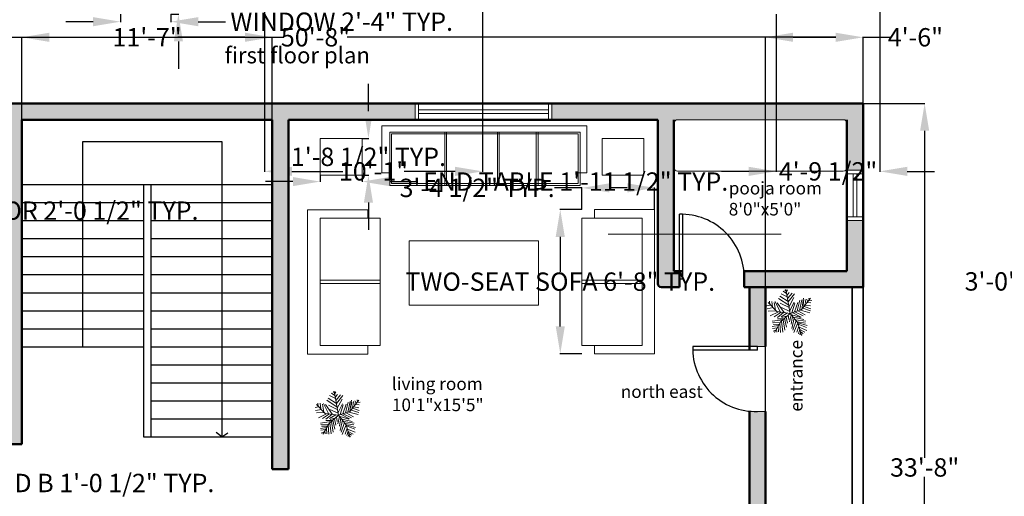
# Model space of a CAD drawing. Units: inches. Extents: x -2 to 7298, y -2 to 4583.
# Tile 3 of 6: x 6252 to 6799, y 3880 to 4144. Entities that reach past the tile are written whole.
import ezdxf

# ---------------------------------------------------------------- set-up
doc = ezdxf.new("R2010")
doc.units = ezdxf.units.IN
doc.header["$MEASUREMENT"] = 0
doc.linetypes.add('ACAD_ISO02W100', pattern=[15, 12, -3])
for name, color, linetype, lineweight in [('A-ANNO-DIMS', 2, 'Continuous', 18), ('A-ANNO-TEXT', 7, 'Continuous', 25), ('A-AREA-IDEN', 7, 'Continuous', 18), ('A-DOOR', 4, 'Continuous', 25), ('A-FLOR-CASE', 30, 'Continuous', 18), ('A-FLOR-STRS', 7, 'Continuous', 25), ('A-FURN', 8, 'Continuous', 18), ('A-GLAZ', 4, 'Continuous', 18), ('A-PLAN-REFR', 8, 'Continuous', 13), ('A-WALL', 7, 'Continuous', 50), ('A-WALL-HIDN', 7, 'ACAD_ISO02W100', 18), ('A-WALL-PATT', 18, 'Continuous', 13), ('C-PROP', 7, 'Continuous', 35), ('L-PLNT', 3, 'Continuous', 13)]:
    doc.layers.add(name, color=color, linetype=linetype, lineweight=lineweight)
doc.styles.get("Standard").update_dxf_attribs({"font": 'arial.ttf'})
doc.dimstyles.get("Standard").update_dxf_attribs({"dimtxt": 10.18, "dimasz": 15.18, "dimexe": 0.18, "dimexo": 0.0625, "dimgap": 0.09, "dimtad": 0, "dimtih": 1, "dimtoh": 1, "dimdec": 0, "dimzin": 0, "dimdsep": 46, "dimlunit": 3, "dimtxsty": 'Standard', "dimcen": 0.09, "dimadec": 0, "dimazin": 0, "dimtfac": 1, "dimtdec": 0, "dimtofl": 0, "dimtmove": 0, "dimatfit": 3, "dimfxl": 1, "dimtolj": 1, "dimtzin": 0, "dimarcsym": 0})

# ---------------------------------------------------------------- blocks, each defined once
blk = doc.blocks.new('*U11')
for p, q in [((-8.737, 47.138), (-17.069, 52.711)), ((-10.186, 53.64), (-13.084, 55.962)), ((0, 0), (-10.5, 57)), ((-9.099, 51.782), (-6.563, 55.962)), ((-7.65, 43.423), (-2.578, 49.46)), ((-5.839, 35.992), (4.667, 48.067)), ((-31.5, 4.5), (-52.5, 25.5)), ((-48.585, 21.131), (-49.309, 29.026)), ((-43.513, 28.561), (-42.427, 15.558)), ((-38.442, 26.239), (-34.819, 7.663)), ((-35.544, 28.097), (-24.314, 3.947)), ((-14.533, 2.09), (-30.834, 25.31)), ((-3.665, 19.273), (-27.574, 35.527)), ((-5.114, 28.097), (-24.676, 40.636)), ((-24.314, 23.917), (-2.941, 13.7)), ((-7.288, 39.707), (-21.778, 46.673)), ((-5.114, 27.632), (10.463, 46.673)), ((-2.941, 16.486), (8.652, 37.85)), ((-1.129, 6.734), (9.014, 26.704)), ((3.942, 1.625), (11.187, 24.381)), ((10.101, 3.483), (17.708, 26.239)), ((16.259, 5.805), (23.142, 31.348)), ((22.055, 7.198), (27.489, 32.277)), ((27, 9), (48, 36)), ((27.127, 9.056), (31.112, 35.992)), ((31.836, 30.883), (32.561, 16.486)), ((35.096, 32.741), (37.27, 22.524)), ((38.719, 34.134), (41.979, 28.561)), ((40.53, 25.775), (48.862, 24.846)), ((43.791, 29.954), (51.036, 30.883)), ((44.153, 36.456), (45.239, 32.741)), ((-47.498, 19.737), (-55.83, 18.344)), ((-40.615, 13.7), (-55.105, 10.913)), ((-33.37, 6.269), (-52.207, 5.34)), ((-28.299, 3.483), (-47.86, -5.805)), ((-21.416, 3.018), (-38.079, -8.128)), ((0, 0), (-31.5, 4.5)), ((-15.982, 2.09), (-30.11, -9.521)), ((0, 0), (-22.5, -19.5)), ((-6.563, 1.161), (-21.416, -8.128)), ((-20.691, 13.7), (-1.129, 4.876)), ((0, 0), (27, 9)), ((0, 0), (18, -22.5)), ((6.478, 1.625), (26.04, -8.592)), ((11.187, 3.483), (30.749, -5.805)), ((18.07, 5.805), (35.096, -3.483)), ((24.229, 7.663), (46.688, 1.625)), ((29.662, 12.307), (48.137, 6.269)), ((33.285, 16.486), (48.862, 10.913)), ((36.183, 19.737), (48.137, 17.88)), ((-17.431, -15.094), (-42.789, -18.809)), ((-24.314, -21.596), (-42.427, -22.06)), ((-22.5, -19.5), (-37.5, -45)), ((-15.257, -12.772), (-30.11, -12.772)), ((-20.691, -18.345), (-17.793, -44.352)), ((-6.563, -5.805), (-19.967, -9.985)), ((-17.069, -15.094), (-12.721, -40.172)), ((-13.446, -11.378), (-8.737, -32.741)), ((-9.461, -8.592), (-6.201, -23.453)), ((-4.752, -3.483), (-3.665, -14.629)), ((2.493, -3.019), (-1.491, -20.202)), ((1.769, -2.555), (24.229, -9.521)), ((5.029, -6.27), (2.131, -25.775)), ((9.014, -11.378), (3.58, -35.992)), ((14.085, -16.951), (6.478, -40.172)), ((7.565, -9.056), (32.198, -14.629)), ((18.07, -22.524), (8.289, -45.745)), ((12.274, -15.094), (36.907, -18.809)), ((16.259, -19.738), (36.183, -22.989)), ((18, -22.5), (27, -52.5)), ((18.433, -22.524), (40.53, -29.026)), ((-28.299, -29.026), (-42.789, -31.348)), ((-30.834, -34.135), (-42.427, -35.528)), ((-34.457, -39.708), (-40.978, -42.494)), ((-26.849, -26.24), (-40.253, -25.775)), ((-32.646, -36.921), (-31.921, -44.352)), ((-29.023, -30.884), (-27.936, -43.887)), ((-25.038, -23.918), (-22.865, -45.281)), ((20.244, -30.419), (15.897, -44.816)), ((19.157, -25.311), (38.719, -33.206)), ((22.78, -37.85), (19.519, -48.532)), ((21.331, -32.741), (39.081, -40.636)), ((22.78, -38.314), (34.372, -44.816)), ((24.591, -45.745), (23.142, -50.854)), ((24.591, -43.423), (30.749, -47.603)), ((26.764, -49.925), (28.213, -50.854))]:
    blk.add_line(p, q)
blk = doc.blocks.new('WINDOW-72IN')
for p, q in [((-2, 4.5), (-2, -4.5)), ((0, 4.5), (0, -4.5)), ((0, 1), (72, 1)), ((72, 4.5), (72, -4.5)), ((74, 4.5), (74, -4.5)), ((0, -1), (72, -1))]:
    blk.add_line(p, q)
blk = doc.blocks.new('WINDOW-24IN')
for p, q in [((-26, 4.5), (-26, -4.5)), ((-24, 4.5), (-24, -4.5)), ((-24, 1), (0, 1)), ((0, 4.5), (0, -4.5)), ((2, 4.5), (2, -4.5)), ((-24, -1), (0, -1))]:
    blk.add_line(p, q)
blk = doc.blocks.new('DOOR-SWING-36IN')
for p, q in [((0, 0), (0, 36)), ((2, 0), (2, 36)), ((2, 0), (0, 0))]:
    blk.add_line(p, q)
blk.add_arc((1, 1), 35.01, 358.3634, 91.6366)
blk = doc.blocks.new('LIVING-END-TABLE')
blk.add_lwpolyline([(0, 20.48), (0, 20.48), (23.29, 20.48), (23.29, 20.48), (23.29, 0), (23.29, 0), (0, 0), (0, 0)], close=True)
blk = doc.blocks.new('SOFA-TWO-SEAT')
for p, q in [((33.34, 80.03), (0, 80.03)), ((0, 80.03), (0, 0)), ((33.34, 75.45), (33.34, 80.03)), ((40.32, 41.12), (6.92, 41.12)), ((40.32, 39.12), (6.92, 39.12)), ((0, 0), (33.34, 0)), ((33.34, 0), (33.34, 4.8))]:
    blk.add_line(p, q)
blk.add_lwpolyline([(40.32, 75.45), (40.32, 75.45), (6.92, 75.45), (6.92, 75.45), (6.92, 4.8), (6.92, 4.8), (40.32, 4.8), (40.32, 4.8)], close=True)
blk = doc.blocks.new('*D39')
at = {"layer": 'A-ANNO-DIMS', "color": 0, "lineweight": -2, "transparency": 16777216}
for p, q in [((6293.09, 4143.28), (6277.91, 4143.28)), ((6308.27, 4147.41), (6308.27, 4143.1)), ((6336.27, 4147.41), (6336.27, 4143.1)), ((6351.45, 4143.28), (6366.63, 4143.28))]:
    blk.add_line(p, q, dxfattribs=at)
at = {"layer": 'A-ANNO-DIMS', "color": 0, "transparency": 16777216}
for points in [[(6293.09, 4145.81), (6293.09, 4140.75), (6308.27, 4143.28)], [(6351.45, 4145.81), (6351.45, 4140.75), (6336.27, 4143.28)]]:
    blk.add_solid(points, dxfattribs=at)
at = {"layer": 'Defpoints', "color": 0, "transparency": 16777216}
for p in [(6308.27, 4147.48), (6336.27, 4147.48), (6336.27, 4143.28)]:
    blk.add_point(p, dxfattribs=at)
at = {"layer": 'A-ANNO-DIMS', "color": 0, "transparency": 16777216, "insert": (6431.13, 4143.28), "char_height": 10.18, "attachment_point": 5}
blk.add_mtext('\\A1;WINDOW 2\'-4" TYP.', dxfattribs=at)
blk = doc.blocks.new('*D40')
at = {"layer": 'A-ANNO-DIMS', "color": 0, "lineweight": -2, "transparency": 16777216}
for p, q in [((6340.47, 4171.66), (6340.47, 4186.84)), ((6340.47, 4186.84), (6355.65, 4186.84)), ((6336.33, 4156.48), (6340.65, 4156.48)), ((6336.33, 4147.48), (6340.65, 4147.48)), ((6340.47, 4132.3), (6340.47, 4117.12))]:
    blk.add_line(p, q, dxfattribs=at)
at = {"layer": 'A-ANNO-DIMS', "color": 0, "transparency": 16777216}
for points in [[(6337.94, 4171.66), (6343, 4171.66), (6340.47, 4156.48)], [(6337.94, 4132.3), (6343, 4132.3), (6340.47, 4147.48)]]:
    blk.add_solid(points, dxfattribs=at)
at = {"layer": 'Defpoints', "color": 0, "transparency": 16777216}
for p in [(6336.27, 4156.48), (6340.47, 4156.48), (6336.27, 4147.48)]:
    blk.add_point(p, dxfattribs=at)
at = {"layer": 'A-ANNO-DIMS', "color": 0, "transparency": 16777216, "insert": (6386.76, 4186.84), "char_height": 10.18, "attachment_point": 5}
blk.add_mtext('\\A1;0\'-9" TYP.', dxfattribs=at)
blk = doc.blocks.new('*D43')
at = {"layer": 'A-ANNO-DIMS', "color": 0, "lineweight": -2, "transparency": 16777216}
for p, q in [((6151.67, 4038.42), (6136.49, 4038.42)), ((6166.85, 4034.84), (6166.85, 4038.6)), ((6191.14, 4034.84), (6191.14, 4038.6)), ((6206.32, 4038.42), (6221.5, 4038.42))]:
    blk.add_line(p, q, dxfattribs=at)
at = {"layer": 'A-ANNO-DIMS', "color": 0, "transparency": 16777216}
for points in [[(6151.67, 4040.95), (6151.67, 4035.89), (6166.85, 4038.42)], [(6206.32, 4040.95), (6206.32, 4035.89), (6191.14, 4038.42)]]:
    blk.add_solid(points, dxfattribs=at)
at = {"layer": 'Defpoints', "color": 0, "transparency": 16777216}
for p in [(6166.85, 4034.78), (6191.14, 4038.42), (6191.14, 4034.78)]:
    blk.add_point(p, dxfattribs=at)
at = {"layer": 'A-ANNO-DIMS', "color": 0, "transparency": 16777216, "insert": (6287.53, 4038.42), "char_height": 10.18, "attachment_point": 5}
blk.add_mtext('\\A1;DOOR 2\'-0 1/2" TYP.', dxfattribs=at)
blk = doc.blocks.new('*D51')
at = {"layer": 'A-ANNO-DIMS', "color": 0, "lineweight": -2, "transparency": 16777216}
for p, q in [((6419.19, 4057.99), (6419.19, 4054.38)), ((6442.48, 4057.99), (6442.48, 4054.38)), ((6404.01, 4054.56), (6388.83, 4054.56)), ((6457.66, 4054.56), (6472.84, 4054.56))]:
    blk.add_line(p, q, dxfattribs=at)
at = {"layer": 'A-ANNO-DIMS', "color": 0, "transparency": 16777216}
for points in [[(6404.01, 4057.09), (6404.01, 4052.03), (6419.19, 4054.56)], [(6457.66, 4057.09), (6457.66, 4052.03), (6442.48, 4054.56)]]:
    blk.add_solid(points, dxfattribs=at)
at = {"layer": 'Defpoints', "color": 0, "transparency": 16777216}
for p in [(6419.19, 4058.06), (6442.48, 4058.06), (6442.48, 4054.56)]:
    blk.add_point(p, dxfattribs=at)
at = {"layer": 'A-ANNO-DIMS', "color": 0, "transparency": 16777216, "insert": (6560.99, 4054.56), "char_height": 10.18, "attachment_point": 5}
blk.add_mtext('\\A1;END TABLE 1\'-11 1/2" TYP.', dxfattribs=at)
blk = doc.blocks.new('*D52')
at = {"layer": 'A-ANNO-DIMS', "color": 0, "lineweight": -2, "transparency": 16777216}
for p, q in [((6445.97, 4093.71), (6445.97, 4108.89)), ((6442.54, 4078.53), (6446.15, 4078.53)), ((6442.54, 4058.06), (6446.15, 4058.06)), ((6445.97, 4042.88), (6445.97, 4027.7))]:
    blk.add_line(p, q, dxfattribs=at)
at = {"layer": 'A-ANNO-DIMS', "color": 0, "transparency": 16777216}
for points in [[(6443.44, 4093.71), (6448.5, 4093.71), (6445.97, 4078.53)], [(6443.44, 4042.88), (6448.5, 4042.88), (6445.97, 4058.06)]]:
    blk.add_solid(points, dxfattribs=at)
at = {"layer": 'Defpoints', "color": 0, "transparency": 16777216}
for p in [(6442.48, 4078.53), (6445.97, 4078.53), (6442.48, 4058.06)]:
    blk.add_point(p, dxfattribs=at)
at = {"layer": 'A-ANNO-DIMS', "color": 0, "transparency": 16777216, "insert": (6445.97, 4068.29), "char_height": 10.18, "attachment_point": 5}
blk.add_mtext('\\A1;1\'-8 1/2" TYP.', dxfattribs=at)
blk = doc.blocks.new('*D55')
at = {"layer": 'A-ANNO-DIMS', "color": 0, "lineweight": -2, "transparency": 16777216}
for p, q in [((6110.57, 3887.28), (6095.39, 3887.28)), ((6125.75, 3889.11), (6125.75, 3887.1)), ((6138.34, 3889.11), (6138.34, 3887.1)), ((6153.52, 3887.28), (6168.7, 3887.28))]:
    blk.add_line(p, q, dxfattribs=at)
at = {"layer": 'A-ANNO-DIMS', "color": 0, "transparency": 16777216}
for points in [[(6110.57, 3889.81), (6110.57, 3884.75), (6125.75, 3887.28)], [(6153.52, 3889.81), (6153.52, 3884.75), (6138.34, 3887.28)]]:
    blk.add_solid(points, dxfattribs=at)
at = {"layer": 'Defpoints', "color": 0, "transparency": 16777216}
for p in [(6125.75, 3889.17), (6138.34, 3889.17), (6138.34, 3887.28)]:
    blk.add_point(p, dxfattribs=at)
at = {"layer": 'A-ANNO-DIMS', "color": 0, "transparency": 16777216, "insert": (6266.35, 3887.28), "char_height": 10.18, "attachment_point": 5}
blk.add_mtext('\\A1;NIGHTSTAND B 1\'-0 1/2" TYP.', dxfattribs=at)
blk = doc.blocks.new('*D57')
at = {"layer": 'A-ANNO-DIMS', "color": 0, "lineweight": -2, "transparency": 16777216}
for p, q in [((6564.4, 4039.04), (6552.27, 4039.04)), ((6552.45, 4023.86), (6552.45, 4004.38)), ((6552.45, 3974.19), (6552.45, 3993.67)), ((6564.4, 3959.01), (6552.27, 3959.01))]:
    blk.add_line(p, q, dxfattribs=at)
at = {"layer": 'A-ANNO-DIMS', "color": 0, "transparency": 16777216}
for points in [[(6549.92, 4023.86), (6554.98, 4023.86), (6552.45, 4039.04)], [(6549.92, 3974.19), (6554.98, 3974.19), (6552.45, 3959.01)]]:
    blk.add_solid(points, dxfattribs=at)
at = {"layer": 'Defpoints', "color": 0, "transparency": 16777216}
for p in [(6564.46, 4039.04), (6552.45, 3959.01), (6564.46, 3959.01)]:
    blk.add_point(p, dxfattribs=at)
at = {"layer": 'A-ANNO-DIMS', "color": 0, "transparency": 16777216, "insert": (6552.45, 3999.03), "char_height": 10.18, "attachment_point": 5}
blk.add_mtext('\\A1;TWO-SEAT SOFA 6\'-8" TYP.', dxfattribs=at)
blk = doc.blocks.new('*D58')
at = {"layer": 'A-ANNO-DIMS', "color": 0, "lineweight": -2, "transparency": 16777216}
for p, q in [((6564.46, 4051.05), (6549.28, 4051.05)), ((6564.46, 4039.1), (6564.46, 4051.23)), ((6589.6, 4051.05), (6579.64, 4051.05)), ((6604.78, 4039.1), (6604.78, 4051.23))]:
    blk.add_line(p, q, dxfattribs=at)
at = {"layer": 'A-ANNO-DIMS', "color": 0, "transparency": 16777216}
for points in [[(6579.64, 4053.58), (6579.64, 4048.52), (6564.46, 4051.05)], [(6589.6, 4053.58), (6589.6, 4048.52), (6604.78, 4051.05)]]:
    blk.add_solid(points, dxfattribs=at)
at = {"layer": 'Defpoints', "color": 0, "transparency": 16777216}
for p in [(6564.46, 4051.05), (6564.46, 4039.04), (6604.78, 4039.04)]:
    blk.add_point(p, dxfattribs=at)
at = {"layer": 'A-ANNO-DIMS', "color": 0, "transparency": 16777216, "insert": (6506.31, 4051.05), "char_height": 10.18, "attachment_point": 5}
blk.add_mtext('\\A1;3\'-4 1/2" TYP.', dxfattribs=at)
blk = doc.blocks.new('*D63')
at = {"layer": 'A-ANNO-DIMS', "color": 0, "lineweight": -2, "transparency": 16777216}
for p, q in [((6253.58, 4088.97), (6253.58, 4134.81)), ((6268.76, 4134.63), (6305.98, 4134.63)), ((6377.4, 4134.63), (6340.17, 4134.63)), ((6392.58, 4088.97), (6392.58, 4134.81))]:
    blk.add_line(p, q, dxfattribs=at)
at = {"layer": 'A-ANNO-DIMS', "color": 0, "transparency": 16777216}
for points in [[(6268.76, 4137.16), (6268.76, 4132.1), (6253.58, 4134.63)], [(6377.4, 4137.16), (6377.4, 4132.1), (6392.58, 4134.63)]]:
    blk.add_solid(points, dxfattribs=at)
at = {"layer": 'Defpoints', "color": 0, "transparency": 16777216}
for p in [(6392.58, 4134.63), (6253.58, 4088.9), (6392.58, 4088.9)]:
    blk.add_point(p, dxfattribs=at)
at = {"layer": 'A-ANNO-DIMS', "color": 0, "transparency": 16777216, "insert": (6323.08, 4134.63), "char_height": 10.18, "attachment_point": 5}
blk.add_mtext('\\A1;11\'-7"', dxfattribs=at)
blk = doc.blocks.new('*D64')
at = {"layer": 'A-ANNO-DIMS', "color": 0, "lineweight": -2, "transparency": 16777216}
for p, q in [((6112.58, 4097.97), (6112.58, 4134.81)), ((6127.76, 4134.63), (6399, 4134.63)), ((6705.4, 4134.63), (6434.15, 4134.63)), ((6720.58, 4097.97), (6720.58, 4134.81))]:
    blk.add_line(p, q, dxfattribs=at)
at = {"layer": 'A-ANNO-DIMS', "color": 0, "transparency": 16777216}
for points in [[(6127.76, 4137.16), (6127.76, 4132.1), (6112.58, 4134.63)], [(6705.4, 4137.16), (6705.4, 4132.1), (6720.58, 4134.63)]]:
    blk.add_solid(points, dxfattribs=at)
at = {"layer": 'Defpoints', "color": 0, "transparency": 16777216}
for p in [(6720.58, 4134.63), (6112.58, 4097.9), (6720.58, 4097.9)]:
    blk.add_point(p, dxfattribs=at)
at = {"layer": 'A-ANNO-DIMS', "color": 0, "transparency": 16777216, "insert": (6416.58, 4134.63), "char_height": 10.18, "attachment_point": 5}
blk.add_mtext('\\A1;50\'-8"', dxfattribs=at)
blk = doc.blocks.new('*D65')
at = {"layer": 'A-ANNO-DIMS', "color": 0, "lineweight": -2, "transparency": 16777216}
for p, q in [((6720.64, 4097.9), (6754.91, 4097.9)), ((6754.73, 4082.72), (6754.73, 3901.2)), ((6754.73, 3709.08), (6754.73, 3890.61)), ((6666.54, 3693.9), (6754.91, 3693.9))]:
    blk.add_line(p, q, dxfattribs=at)
at = {"layer": 'A-ANNO-DIMS', "color": 0, "transparency": 16777216}
for points in [[(6752.2, 4082.72), (6757.26, 4082.72), (6754.73, 4097.9)], [(6752.2, 3709.08), (6757.26, 3709.08), (6754.73, 3693.9)]]:
    blk.add_solid(points, dxfattribs=at)
at = {"layer": 'Defpoints', "color": 0, "transparency": 16777216}
for p in [(6720.58, 4097.9), (6754.73, 4097.9), (6666.47, 3693.9)]:
    blk.add_point(p, dxfattribs=at)
at = {"layer": 'A-ANNO-DIMS', "color": 0, "transparency": 16777216, "insert": (6754.73, 3895.9), "char_height": 10.18, "attachment_point": 5}
blk.add_mtext('\\A1;33\'-8"', dxfattribs=at)
blk = doc.blocks.new('*D68')
at = {"layer": 'A-ANNO-DIMS', "color": 0, "lineweight": -2, "transparency": 16777216}
for p, q in [((6666.47, 3693.97), (6666.47, 4134.81)), ((6681.65, 4134.63), (6705.4, 4134.63)), ((6720.58, 3594.45), (6720.58, 4134.81)), ((6720.58, 4134.63), (6735.76, 4134.63))]:
    blk.add_line(p, q, dxfattribs=at)
at = {"layer": 'A-ANNO-DIMS', "color": 0, "transparency": 16777216}
for points in [[(6681.65, 4137.16), (6681.65, 4132.1), (6666.47, 4134.63)], [(6705.4, 4137.16), (6705.4, 4132.1), (6720.58, 4134.63)]]:
    blk.add_solid(points, dxfattribs=at)
at = {"layer": 'Defpoints', "color": 0, "transparency": 16777216}
for p in [(6720.58, 4134.63), (6666.47, 3693.9), (6720.58, 3594.39)]:
    blk.add_point(p, dxfattribs=at)
at = {"layer": 'A-ANNO-DIMS', "color": 0, "transparency": 16777216, "insert": (6749.58, 4134.63), "char_height": 10.18, "attachment_point": 5}
blk.add_mtext('\\A1;4\'-6"', dxfattribs=at)
blk = doc.blocks.new('*D69')
at = {"layer": 'A-ANNO-DIMS', "color": 0, "lineweight": -2, "transparency": 16777216}
for p, q in [((6729.865325, 4148.84694), (6729.865325, 4060.046544)), ((6672.267047, 4147.414044), (6672.267047, 4060.046544)), ((6657.087047, 4060.226544), (6641.907047, 4060.226544)), ((6745.045325, 4060.226544), (6760.225325, 4060.226544))]:
    blk.add_line(p, q, dxfattribs=at)
at = {"layer": 'A-ANNO-DIMS', "color": 0, "transparency": 16777216}
for points in [[(6657.087047, 4062.756544), (6657.087047, 4057.696544), (6672.267047, 4060.226544)], [(6745.045325, 4062.756544), (6745.045325, 4057.696544), (6729.865325, 4060.226544)]]:
    blk.add_solid(points, dxfattribs=at)
at = {"layer": 'Defpoints', "color": 0, "transparency": 16777216}
for p in [(6729.865325, 4148.90944), (6672.267047, 4147.476544), (6729.865325, 4060.226544)]:
    blk.add_point(p, dxfattribs=at)
at = {"layer": 'A-ANNO-DIMS', "color": 0, "transparency": 16777216, "insert": (6701.066186, 4060.226544), "char_height": 10.18, "attachment_point": 5}
blk.add_mtext('\\A1;4\'-9 1/2"', dxfattribs=at)
blk = doc.blocks.new('*D71')
at = {"layer": 'A-ANNO-DIMS', "color": 0, "lineweight": -2, "transparency": 16777216}
for p, q in [((6509.27, 4416.41), (6509.27, 4060.05)), ((6388.27, 4404.41), (6388.27, 4060.05)), ((6403.45, 4060.23), (6431.67, 4060.23)), ((6494.09, 4060.23), (6465.86, 4060.23))]:
    blk.add_line(p, q, dxfattribs=at)
at = {"layer": 'A-ANNO-DIMS', "color": 0, "transparency": 16777216}
for points in [[(6403.45, 4062.76), (6403.45, 4057.7), (6388.27, 4060.23)], [(6494.09, 4062.76), (6494.09, 4057.7), (6509.27, 4060.23)]]:
    blk.add_solid(points, dxfattribs=at)
at = {"layer": 'Defpoints', "color": 0, "transparency": 16777216}
for p in [(6509.27, 4416.48), (6388.27, 4404.48), (6509.27, 4060.23)]:
    blk.add_point(p, dxfattribs=at)
at = {"layer": 'A-ANNO-DIMS', "color": 0, "transparency": 16777216, "insert": (6448.77, 4060.23), "char_height": 10.18, "attachment_point": 5}
blk.add_mtext('\\A1;10\'-1"', dxfattribs=at)
blk = doc.blocks.new('*D84')
at = {"layer": 'A-ANNO-DIMS', "color": 0, "lineweight": -2, "transparency": 16777216}
for p, q in [((6960.88, 4050.44), (6820.87, 4050.44)), ((6821.05, 4035.26), (6821.05, 4029.51)), ((7076.44, 4014.33), (6820.87, 4014.33)), ((6821.05, 4014.33), (6821.05, 3999.15)), ((6821.05, 3999.15), (6805.87, 3999.15))]:
    blk.add_line(p, q, dxfattribs=at)
at = {"layer": 'A-ANNO-DIMS', "color": 0, "transparency": 16777216}
for points in [[(6818.52, 4035.26), (6823.58, 4035.26), (6821.05, 4050.44)], [(6818.52, 4029.51), (6823.58, 4029.51), (6821.05, 4014.33)]]:
    blk.add_solid(points, dxfattribs=at)
at = {"layer": 'Defpoints', "color": 0, "transparency": 16777216}
for p in [(6960.94, 4050.44), (6821.05, 4014.33), (7076.5, 4014.33)]:
    blk.add_point(p, dxfattribs=at)
at = {"layer": 'A-ANNO-DIMS', "color": 0, "transparency": 16777216, "insert": (6792.26, 3999.15), "char_height": 10.18, "attachment_point": 5}
blk.add_mtext('\\A1;3\'-0"', dxfattribs=at)

msp = doc.modelspace()

# ---------------------------------------------------------------- hatches: boundary and pattern name
at = {"layer": 'A-WALL-PATT'}
h = msp.add_hatch(color=256, dxfattribs=at)
h.dxf.hatch_style = 1
h.paths.add_polyline_path([(6253.58, 3872.9), (6244.58, 3872.9), (6244.58, 3869.9), (6121.58, 3869.9), (6121.58, 3906.9), (6112.58, 3906.9), (6112.58, 3860.9), (6244.58, 3860.9), (6244.58, 3693.9), (6289.08, 3693.9), (6289.08, 3702.9), (6253.58, 3702.9), (6253.58, 3830.9), (6337.58, 3830.9), (6337.58, 3833.4, -0.014283), (6337.58, 3835.4), (6337.58, 3839.9), (6253.58, 3839.9)])
h.paths.add_polyline_path([(6385.58, 3839.9), (6373.58, 3839.9), (6373.58, 3830.9), (6376.58, 3830.9), (6376.58, 3702.9), (6341.08, 3702.9), (6341.08, 3693.9), (6410.08, 3693.9), (6410.08, 3702.9), (6385.58, 3702.9)])
h.paths.add_polyline_path([(6519.58, 3864.9), (6557.19, 3864.9), (6557.19, 3873.9), (6510.58, 3873.9), (6510.58, 3839.9), (6510.58, 3702.9), (6486.08, 3702.9), (6486.08, 3693.9), (6562.53, 3693.9), (6562.53, 3702.9), (6519.58, 3702.9)])
h.paths.add_polyline_path([(6666.47, 3745.9), (6657.47, 3745.9), (6657.47, 3702.9), (6614.53, 3702.9), (6614.53, 3693.9), (6666.47, 3693.9)])
h.paths.add_polyline_path([(6666.47, 3926.97), (6661.97, 3926.97, -0.014283), (6659.97, 3926.97), (6657.47, 3926.97), (6657.47, 3873.9), (6606.04, 3873.9), (6606.04, 3864.9), (6657.47, 3864.9), (6657.47, 3821.9), (6666.47, 3821.9)])
h.paths.add_polyline_path([(6720.58, 4097.9), (6547.84, 4097.9), (6547.84, 4088.9), (6606.58, 4088.9), (6606.58, 3997.9, 0.414214), (6608.58, 3995.9), (6618.58, 3995.9), (6618.58, 4004.9), (6615.58, 4004.9), (6615.58, 4088.9), (6711.58, 4088.9), (6711.58, 4060.9), (6720.58, 4060.9)])
h.paths.add_polyline_path([(6720.58, 4032.9), (6711.58, 4032.9), (6711.58, 4004.9), (6654.58, 4004.9), (6654.58, 4002.4, -0.014283), (6654.58, 4000.4), (6654.58, 3995.9), (6711.58, 3995.9), (6720.58, 3995.9)], flags=17)
h.paths.add_polyline_path([(6471.84, 4097.9), (6233.45, 4097.9), (6233.45, 4088.9), (6244.58, 4088.9), (6244.58, 4004.9), (6244.58, 3995.9), (6244.58, 3908.9), (6247.08, 3908.9, -0.014283), (6249.08, 3908.9), (6253.58, 3908.9), (6253.58, 3995.9), (6253.58, 4088.9), (6392.58, 4088.9), (6392.58, 4004.9), (6392.58, 3995.9), (6392.58, 3894.9), (6401.58, 3894.9), (6401.58, 3995.9), (6401.58, 4004.9), (6401.58, 4088.9), (6471.84, 4088.9)])
h.paths.add_polyline_path([(6205.45, 4097.9), (6112.58, 4097.9), (6112.58, 4060.9), (6121.58, 4060.9), (6121.58, 4088.9), (6186.64, 4088.9), (6186.64, 4034.49), (6189.14, 4034.49, -0.021729), (6191.14, 4034.49), (6195.64, 4034.49), (6195.64, 4088.9), (6202.58, 4088.9), (6205.45, 4088.9)])
h.paths.add_polyline_path([(6121.58, 3995.9), (6217.58, 3995.9), (6217.58, 4000.4, -0.021729), (6217.58, 4002.4), (6217.58, 4004.9), (6195.64, 4004.9), (6195.64, 4010.49), (6186.64, 4010.49), (6186.64, 4004.9), (6121.58, 4004.9), (6121.58, 4032.9), (6112.58, 4032.9), (6112.58, 3958.9), (6121.58, 3958.9)])
h = msp.add_hatch(color=256, dxfattribs=at)
h.dxf.hatch_style = 1
h.paths.add_polyline_path([(6657.47, 3962.97), (6661.97, 3962.97), (6666.47, 3962.97), (6666.47, 3995.9), (6657.47, 3995.9)])

# ---------------------------------------------------------------- linework, layer by layer
at = {"layer": 'A-DOOR'}
for p, q in [((6661.97, 3962.97), (6625.97, 3962.97)), ((6661.97, 3960.97), (6661.97, 3962.97)), ((6661.97, 3960.97), (6625.97, 3960.97))]:
    msp.add_line(p, q, dxfattribs=at)
msp.add_arc((6660.97, 3961.97), 35.01, 178.3634, 271.6366, dxfattribs=at)
at = {"layer": 'A-FLOR-CASE'}
msp.add_lwpolyline([(6615.58, 4086.9, -0.414214), (6617.58, 4088.9), (6709.58, 4088.9, -0.414214), (6711.58, 4086.9), (6711.58, 4062.28, -0.414214), (6709.58, 4060.28), (6617.58, 4060.28, -0.414214), (6615.58, 4062.28)], format="xyb", close=True, dxfattribs=at)
at = {"layer": 'A-FLOR-STRS'}
for p, q in [((6287.33, 3962.9), (6287.33, 4076.77)), ((6287.33, 4076.77), (6364.59, 4076.77)), ((6364.59, 4076.77), (6364.59, 3912.9)), ((6253.58, 4052.9), (6392.58, 4052.9)), ((6321.08, 4052.9), (6321.08, 3912.9)), ((6325.08, 4052.9), (6325.08, 3912.9)), ((6253.58, 4042.9), (6321.08, 4042.9)), ((6325.08, 4042.9), (6392.58, 4042.9)), ((6253.58, 4032.9), (6321.08, 4032.9)), ((6325.08, 4032.9), (6392.58, 4032.9)), ((6253.58, 4022.9), (6321.08, 4022.9)), ((6325.08, 4022.9), (6392.58, 4022.9)), ((6253.58, 4012.9), (6321.08, 4012.9)), ((6325.08, 4012.9), (6392.58, 4012.9)), ((6253.58, 4002.9), (6321.08, 4002.9)), ((6325.08, 4002.9), (6392.58, 4002.9)), ((6253.58, 3992.9), (6321.08, 3992.9)), ((6325.08, 3992.9), (6392.58, 3992.9)), ((6253.58, 3982.9), (6321.08, 3982.9)), ((6325.08, 3982.9), (6392.58, 3982.9)), ((6253.58, 3972.9), (6321.08, 3972.9)), ((6325.08, 3972.9), (6392.58, 3972.9)), ((6253.58, 3962.9), (6321.08, 3962.9)), ((6325.08, 3962.9), (6392.58, 3962.9)), ((6325.08, 3952.9), (6392.58, 3952.9)), ((6325.08, 3942.9), (6392.58, 3942.9)), ((6325.08, 3932.9), (6392.58, 3932.9)), ((6325.08, 3922.9), (6392.58, 3922.9)), ((6364.59, 3912.9), (6361.47, 3915.28)), ((6364.59, 3912.9), (6367.89, 3915.07)), ((6321.08, 3912.9), (6392.58, 3912.9))]:
    msp.add_line(p, q, dxfattribs=at)
at = {"layer": 'A-FURN'}
for p, q in [((6453.34, 4059.4), (6453.34, 4085.58)), ((6453.34, 4085.58), (6567.13, 4085.58)), ((6567.13, 4085.58), (6567.13, 4059.4)), ((6488.34, 4082.01), (6488.34, 4052.46)), ((6489.34, 4082.01), (6489.34, 4052.46)), ((6517.59, 4082.01), (6517.59, 4052.46)), ((6518.59, 4082.01), (6518.59, 4052.46)), ((6539.1, 4082.01), (6539.1, 4052.46)), ((6540.1, 4082.01), (6540.1, 4052.46)), ((6457.78, 4059.4), (6453.34, 4059.4)), ((6457.78, 4059.4), (6457.78, 4059.4)), ((6567.13, 4059.4), (6562.41, 4059.4))]:
    msp.add_line(p, q, dxfattribs=at)
for points in [[(6457.78, 4082.01), (6457.78, 4082.01), (6563.41, 4082.01), (6563.41, 4082.01), (6563.41, 4052.46), (6563.41, 4052.46), (6457.78, 4052.46), (6457.78, 4052.46)], [(6458.78, 4081.01), (6562.41, 4081.01), (6562.41, 4053.46), (6458.78, 4053.46)], [(6468.65, 4021.6), (6468.65, 4021.6), (6540.37, 4021.6), (6540.37, 4021.6), (6540.37, 3986.02), (6540.37, 3986.02), (6468.65, 3986.02), (6468.65, 3986.02)]]:
    msp.add_lwpolyline(points, close=True, dxfattribs=at)
at = {"layer": 'A-PLAN-REFR'}
msp.add_line((6579.13, 4025.31), (6675.13, 4025.31), dxfattribs=at)
at = {"layer": 'A-WALL'}
for p, q in [((6112.58, 4097.9), (6720.58, 4097.9)), ((6720.58, 4097.9), (6720.58, 3995.9)), ((6253.58, 4088.9), (6392.58, 4088.9)), ((6253.58, 3995.9), (6253.58, 4088.9)), ((6392.58, 4088.9), (6392.58, 4004.9)), ((6401.58, 4088.9), (6401.58, 4004.9)), ((6401.58, 4088.9), (6476.58, 4088.9)), ((6476.58, 4088.9), (6485.58, 4088.9)), ((6485.58, 4088.9), (6606.58, 4088.9)), ((6606.58, 4088.9), (6606.58, 3997.9)), ((6615.58, 4088.9), (6615.58, 4004.9)), ((6711.58, 4088.9), (6711.58, 4004.9)), ((6392.58, 4004.9), (6392.58, 3995.9)), ((6401.58, 4004.9), (6401.58, 3995.9)), ((6615.58, 4004.9), (6620.58, 4004.9)), ((6618.58, 4004.9), (6618.58, 3995.9)), ((6654.42, 4004.9), (6711.58, 4004.9)), ((6654.58, 4004.9), (6654.58, 3995.9)), ((6253.58, 3908.9), (6253.58, 3995.9)), ((6392.58, 3995.9), (6392.58, 3894.9)), ((6401.58, 3995.9), (6401.58, 3894.9)), ((6608.58, 3995.9), (6618.58, 3995.9)), ((6654.58, 3995.9), (6711.58, 3995.9)), ((6657.47, 3995.9), (6657.47, 3960.97)), ((6666.47, 3995.9), (6666.47, 3962.97)), ((6666.47, 3995.9), (6720.58, 3995.9)), ((6657.47, 3927.13), (6657.47, 3873.9)), ((6666.47, 3926.97), (6666.47, 3693.9)), ((6244.58, 3908.9), (6253.58, 3908.9)), ((6392.58, 3894.9), (6401.58, 3894.9))]:
    msp.add_line(p, q, dxfattribs=at)
msp.add_arc((6608.58, 3997.9), 2, 180, 270, dxfattribs=at)
at = {"layer": 'A-WALL-HIDN'}
for p, q in [((6666.47, 3962.97), (6657.47, 3962.97)), ((6666.47, 3926.97), (6657.47, 3926.97))]:
    msp.add_line(p, q, dxfattribs=at)
at = {"layer": 'C-PROP'}
for p, q in [((6714.58, 3995.9), (6714.58, 3600.39)), ((6720.58, 3995.9), (6720.58, 3594.39))]:
    msp.add_line(p, q, dxfattribs=at)

# ---------------------------------------------------------------- block references
at = {"layer": 'A-DOOR'}
msp.add_blockref('DOOR-SWING-36IN', (6618.58, 4000.4), dxfattribs=at)
at = {"layer": 'A-FURN'}
for name, p in [('LIVING-END-TABLE', (6419.19, 4058.05)), ('LIVING-END-TABLE', (6575.62, 4058.05)), ('SOFA-TWO-SEAT', (6412.22, 3958.79))]:
    msp.add_blockref(name, p, dxfattribs=at)
at = {"layer": 'A-FURN', "rotation": 180}
msp.add_blockref('SOFA-TWO-SEAT', (6604.78, 4039.04), dxfattribs=at)
at = {"layer": 'A-GLAZ'}
for name, p, rotation in [('WINDOW-72IN', (6545.84, 4093.4), 180), ('WINDOW-24IN', (6716.08, 4058.9), 90.00000000000284)]:
    msp.add_blockref(name, p, dxfattribs=dict(at, rotation=rotation))
at = {"layer": 'L-PLNT', "xscale": 0.2336039447018575, "yscale": 0.2336039447018575, "zscale": 0.2336039447018575}
for p in [(6680.12, 3981.4), (6429.38, 3924.89)]:
    msp.add_blockref('*U11', p, dxfattribs=at)

# ---------------------------------------------------------------- texts
at = {"layer": 'A-ANNO-TEXT', "insert": (6366.16, 4129.16), "char_height": 9, "attachment_point": 1}
msp.add_mtext_dynamic_manual_height_columns('first floor plan', width=436.0251, gutter_width=1, heights=[0], dxfattribs=at)
at = {"layer": 'A-AREA-IDEN', "char_height": 7, "attachment_point": 1}
for s, insert in [('pooja room\\P8\'0"x5\'0"', (6645.96, 4054.41)), ('living room\\P10\'1"x15\'5"', (6458.98, 3945.82)), ('north east', (6586.03, 3941.51))]:
    msp.add_mtext_dynamic_manual_height_columns(s, width=127.1277, gutter_width=1, heights=[0], dxfattribs=dict(at, insert=insert))
at = {"layer": 'A-AREA-IDEN', "insert": (6679.95, 3926.87), "char_height": 7, "attachment_point": 1, "rotation": 90}
msp.add_mtext_dynamic_manual_height_columns('entrance', width=127.1277, gutter_width=1, heights=[0], dxfattribs=at)

# ---------------------------------------------------------------- dimensions: what is measured, and where the dimension line sits
at = {"layer": 'A-ANNO-DIMS'}
for base, p1, p2, picture, middle in [((6509.27, 4060.23), (6388.27, 4404.48), (6509.27, 4416.48), '*D71', (6448.77, 4060.23)), ((6729.87, 4060.23), (6672.27, 4147.48), (6729.87, 4148.91), '*D69', (6701.07, 4060.23)), ((6720.58, 4134.63), (6112.58, 4097.9), (6720.58, 4097.9), '*D64', (6416.58, 4134.63)), ((6392.58, 4134.63), (6253.58, 4088.9), (6392.58, 4088.9), '*D63', (6323.08, 4134.63)), ((6720.58, 4134.63), (6666.47, 3693.9), (6720.58, 3594.39), '*D68', (6749.58, 4134.63))]:
    dim = msp.add_linear_dim(base=base, p1=p1, p2=p2, dimstyle='Standard', override={"dimdec": 1, "dimlfac": 1, "dimrnd": 0, "dimzin": 1, "dimdsep": 46, "dimlunit": 4, "dimfrac": 2}, dxfattribs=at)
    dim.commit()
    dim.dimension.update_dxf_attribs({"geometry": picture, "text_midpoint": middle})
for base, p1, p2, angle, text, picture, middle in [((6340.47, 4156.48), (6336.27, 4147.48), (6336.27, 4156.48), 90, '<> TYP.', '*D40', (6386.76, 4186.84)), ((6445.97, 4078.53), (6442.48, 4058.06), (6442.48, 4078.53), 90, '<> TYP.', '*D52', (6445.97, 4068.29)), ((6564.46, 4051.05), (6604.78, 4039.04), (6564.46, 4039.04), 180, '<> TYP.', '*D58', (6506.31, 4051.05)), ((6552.45, 3959.01), (6564.46, 4039.04), (6564.46, 3959.01), 270, 'TWO-SEAT SOFA <> TYP.', '*D57', (6552.45, 3999.03))]:
    dim = msp.add_linear_dim(base=base, p1=p1, p2=p2, angle=angle, text=text, dimstyle='Standard', override={"dimdec": 1, "dimlfac": 1, "dimrnd": 0, "dimzin": 1, "dimdsep": 46, "dimlunit": 4, "dimfrac": 2}, dxfattribs=at)
    dim.commit()
    dim.dimension.update_dxf_attribs({"geometry": picture, "text_midpoint": middle})
for base, p1, p2, text, picture, middle in [((6336.27, 4143.28), (6308.27, 4147.48), (6336.27, 4147.48), 'WINDOW <> TYP.', '*D39', (6431.13, 4143.28)), ((6442.48, 4054.56), (6419.19, 4058.06), (6442.48, 4058.06), 'END TABLE <> TYP.', '*D51', (6560.99, 4054.56)), ((6191.14, 4038.42), (6166.85, 4034.78), (6191.14, 4034.78), 'DOOR <> TYP.', '*D43', (6287.53, 4038.42)), ((6138.34, 3887.28), (6125.75, 3889.17), (6138.34, 3889.17), 'NIGHTSTAND B <> TYP.', '*D55', (6266.35, 3887.28))]:
    dim = msp.add_linear_dim(base=base, p1=p1, p2=p2, text=text, dimstyle='Standard', override={"dimdec": 1, "dimlfac": 1, "dimrnd": 0, "dimzin": 1, "dimdsep": 46, "dimlunit": 4, "dimfrac": 2}, dxfattribs=at)
    dim.commit()
    dim.dimension.update_dxf_attribs({"geometry": picture, "text_midpoint": middle})
for base, p1, p2, picture, middle in [((6754.73, 4097.9), (6666.47, 3693.9), (6720.58, 4097.9), '*D65', (6754.73, 3895.9)), ((6821.05, 4014.33), (6960.94, 4050.44), (7076.5, 4014.33), '*D84', (6792.26, 3999.15))]:
    dim = msp.add_linear_dim(base=base, p1=p1, p2=p2, angle=90, dimstyle='Standard', override={"dimdec": 1, "dimlfac": 1, "dimrnd": 0, "dimzin": 1, "dimdsep": 46, "dimlunit": 4, "dimfrac": 2}, dxfattribs=at)
    dim.commit()
    dim.dimension.update_dxf_attribs({"geometry": picture, "text_midpoint": middle})

doc.saveas('drawing.dxf')
